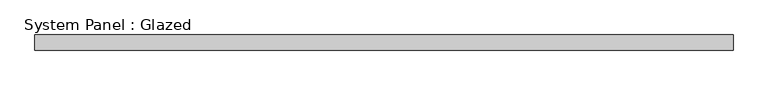
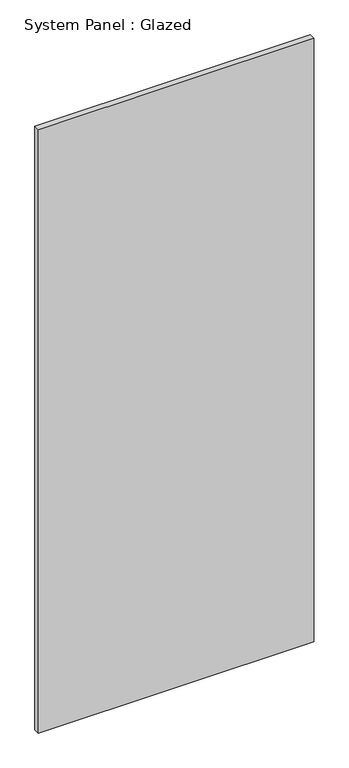
"""IFC4 building model written with IfcOpenShell, lengths in millimetres: plate geometry, System Panel : Glazed."""

from ifc_helpers import new_model, si_unit, origin, origin_with_axes, place, context, project, spatial, polyline, outline, extrude, source, transform, mapped, element, save


def system_panel_glazed_be7f0fdb(model_context):
    return source(origin(), model_context, "Body", "SweptSolid", [
        extrude(outline(polyline([(571.1875873, 19.05), (-571.1875873, 19.05), (-571.1875873, 44.45), (571.1875873, 44.45), (571.1875873, 19.05)])), origin_with_axes(), (0.0, 0.0, 1.0), 2647.95),
    ])


if __name__ == "__main__":
    model = new_model("IFC4")
    model_context = context("Model", 3, world=origin())
    ifc_project = project(units=[si_unit("LENGTHUNIT", "METRE", prefix="MILLI")], contexts=[model_context])
    site = spatial("IfcSite", under=ifc_project)
    building = spatial("IfcBuilding", under=site)
    placement = place(None, origin())
    system_panel_glazed_shape = system_panel_glazed_be7f0fdb(model_context)
    element("IfcPlate", 1, ObjectType="System Panel : Glazed", at=placement, inside=building, context=model_context, shape_type="MappedRepresentation", body=[
        mapped(system_panel_glazed_shape, transform((0.0, 0.0, 0.0), x_axis=(1.0, 0.0, 0.0), y_axis=(0.0, 1.0, 0.0), z_axis=(0.0, 0.0, 1.0))),
    ])
    save(model, "model.ifc")

# Revit data of these elements
# Type "System Panel : Glazed"
#   Construction Type Id = "GSP4R"
#   Analytic Construction = "1/8 in Pilkington single glazing"
#   Visual Light Transmittance = 0.9
#   Solar Heat Gain Coefficient = 0.86
#   Heat Transfer Coefficient (U) = 1.18115 BTU/(h·ft²·°F)
# Element 1 (IfcPlate, "System Panel : Glazed")
#   Materials on its faces: "Glass"
# Materials
#   "Glass": class "Glass", colour RGB 0 128 192, transparency 0.75, Description = "Soda Lime Glass", Cost = 0
